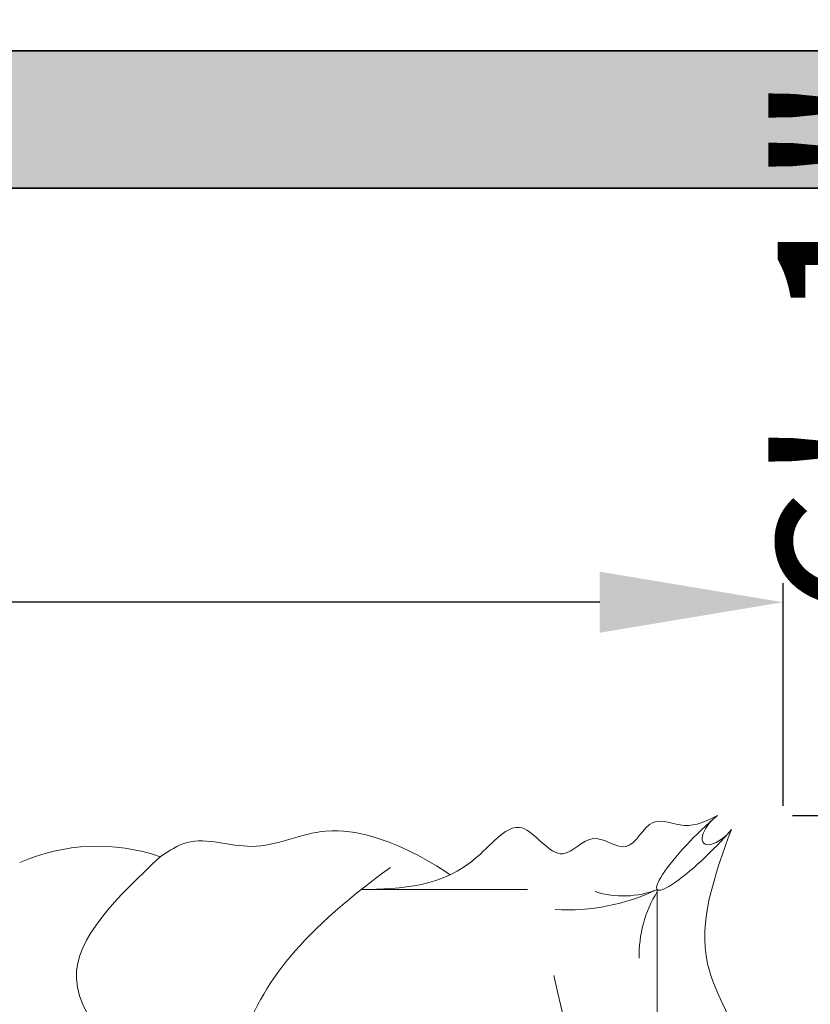
# Model space of a CAD drawing. Units: inches. Extents: x 2083 to 3317, y 1141 to 2115.
# Tile 99 of 256: x 2287 to 2339, y 1958 to 2023. Entities that reach past the tile are written whole.
import ezdxf

# ---------------------------------------------------------------- set-up
doc = ezdxf.new("R2010")
doc.units = ezdxf.units.IN
for name, color, linetype, lineweight in [('A-ANNO-DIMS', 2, 'Continuous', 18), ('A-FURN', 8, 'Continuous', 18), ('A-WALL', 7, 'Continuous', 35), ('www.cadblocksfree.com', 7, 'Continuous', 9)]:
    doc.layers.add(name, color=color, linetype=linetype, lineweight=lineweight)
doc.layers.add('A-WALL-PATT', color=251, linetype='Continuous', lineweight=13, true_color=0x636466)
doc.styles.get("Standard").update_dxf_attribs({"font": 'arial.ttf'})
doc.dimstyles.new('ISO-25', dxfattribs={"dimtxt": 12, "dimasz": 12, "dimexe": 1.25, "dimexo": 0.625, "dimtad": 1, "dimlunit": 3, "dimtxsty": 'Standard', "dimcen": 2.5, "dimadec": 0, "dimazin": 0, "dimtfac": 1, "dimtmove": 0, "dimatfit": 3, "dimfxl": 1, "dimarcsym": 0})

# ---------------------------------------------------------------- blocks, each defined once
blk = doc.blocks.new('bed')
at = {"layer": 'www.cadblocksfree.com', "ltscale": 0.2}
for p, q in [((3426.379, 1399.908), (3426.379, 1410.814)), ((3363.387, 1391.414), (3426.379, 1391.414))]:
    blk.add_line(p, q, dxfattribs=at)
for centre, radius, start, end in [((3416.575, 1428.082), 12.646, 341.02679, 23.77822), ((3438.819, 1397.314), 13.768, 176.75247, 205.37301), ((3432.135, 1393.639), 6.173, 162.64747, 201.1361), ((3422.111, 1384.801), 7.798, 58.00129, 91.65506)]:
    blk.add_arc(centre, radius, start, end, dxfattribs=at)
for centre, major_axis, ratio, start_param, end_param in [((3429.422, 1388.371), (-3.043, 3.043), 0.168252, 4.250342, 8.316029), ((3430.477, 1387.316), (-1.055, 1.055), 0.453532, 4.422107, 8.144264)]:
    blk.add_ellipse(centre, major_axis=major_axis, ratio=ratio, start_param=start_param, end_param=end_param, dxfattribs=at)
for points, knots in [([(3365.512, 1424.213), (3370.519, 1427.004), (3381.149, 1429.825), (3396.214, 1425.866), (3410.541, 1420.654), (3420.273, 1432.695), (3425.882, 1426.771), (3428.534, 1423.97)], [0.099185, 0.099185, 0.099185, 0.099185, 0.523647, 0.927087, 1.289918, 1.564439, 1.810555, 1.810555, 1.810555, 1.810555]), ([(3428.534, 1423.97), (3428.914, 1423.397), (3430.098, 1421.613), (3428.491, 1417.656), (3430.593, 1413.794), (3429.801, 1409.122), (3428.396, 1406.564), (3427.355, 1404.971)], [0, 0, 0, 0, 0.050513, 0.157399, 0.2842023, 0.3628173, 0.5066917, 0.5066917, 0.5066917, 0.5066917]), ([(3362.057, 1409.866), (3363.638, 1413.65), (3372.978, 1421.337), (3389.682, 1406.045), (3402.396, 1419.984), (3416.037, 1420.167), (3423.233, 1415.231), (3427.827, 1408.899)], [0.029901, 0.029901, 0.029901, 0.029901, 0.276967, 0.797115, 1.093669, 1.464666, 1.788489, 1.788489, 1.788489, 1.788489]), ([(3431.237, 1387.473), (3430.882, 1388.172), (3430.205, 1389.505), (3431.478, 1391.985), (3428.294, 1393.194), (3430.501, 1395.689), (3427.558, 1397.866), (3431.841, 1400.386), (3426.535, 1404.33), (3426.443, 1408.152), (3426.379, 1410.814)], [0, 0, 0, 0, 2.267059, 4.324559, 6.685584, 8.878641, 11.121502, 14.300359, 17.755284, 25.682856, 25.682856, 25.682856, 25.682856]), ([(3368.632, 1397.839), (3375.978, 1400.489), (3385.349, 1402.757), (3397.531, 1395.273), (3413.593, 1410.377), (3407.806, 1395.019), (3420.759, 1398.2)], [0.029901, 0.029901, 0.029901, 0.029901, 0.276967, 0.797115, 1.093669, 1.16836, 1.16836, 1.16836, 1.16836]), ([(3430.32, 1386.556), (3427.327, 1387.653), (3422.148, 1389.55), (3414.529, 1384.137), (3405.607, 1387.046), (3396.29, 1386.314), (3386.838, 1381.282), (3377.742, 1390.272), (3370.778, 1384.799), (3364.626, 1383.966), (3363.275, 1388.265), (3360.778, 1387.151), (3359.446, 1386.556)], [0, 0, 0, 0, 8.93042, 15.449194, 25.485629, 34.878505, 43.598887, 54.554403, 64.16647, 67.461673, 70.610457, 74.213583, 74.213583, 74.213583, 74.213583])]:
    blk.add_open_spline(points, degree=3, knots=knots, dxfattribs=at)
blk = doc.blocks.new('*D20')
at = {"layer": 'A-ANNO-DIMS', "color": 0, "lineweight": -2, "transparency": 16777216}
for p, q in [((2244.15, 1971.316), (2244.15, 1985.902)), ((2337.22, 1971.316), (2337.22, 1985.902)), ((2244.15, 1984.652), (2119.159, 1984.652)), ((2325.22, 1984.652), (2256.15, 1984.652))]:
    blk.add_line(p, q, dxfattribs=at)
at = {"layer": 'A-ANNO-DIMS', "color": 0, "transparency": 16777216}
for points in [[(2256.15, 1986.652), (2256.15, 1982.652), (2244.15, 1984.652)], [(2325.22, 1986.652), (2325.22, 1982.652), (2337.22, 1984.652)]]:
    blk.add_solid(points, dxfattribs=at)
at = {"layer": 'Defpoints', "color": 0, "transparency": 16777216}
for p in [(2244.15, 1984.652), (2244.15, 1970.691), (2337.22, 1970.691)]:
    blk.add_point(p, dxfattribs=at)
at = {"layer": 'A-ANNO-DIMS', "color": 0, "transparency": 16777216, "insert": (2175.654, 1991.404), "char_height": 12, "attachment_point": 5}
blk.add_mtext('BED 7\'-9" TYP.', dxfattribs=at)
blk = doc.blocks.new('*D21')
at = {"layer": 'A-ANNO-DIMS', "color": 0, "lineweight": -2, "transparency": 16777216}
for p, q in [((2351.181, 1970.691), (2351.181, 2057.153)), ((2337.845, 1970.691), (2352.431, 1970.691)), ((2351.181, 1909.744), (2351.181, 1958.691)), ((2337.845, 1897.744), (2352.431, 1897.744))]:
    blk.add_line(p, q, dxfattribs=at)
at = {"layer": 'A-ANNO-DIMS', "color": 0, "transparency": 16777216}
for points in [[(2349.181, 1958.691), (2353.181, 1958.691), (2351.181, 1970.691)], [(2349.181, 1909.744), (2353.181, 1909.744), (2351.181, 1897.744)]]:
    blk.add_solid(points, dxfattribs=at)
at = {"layer": 'Defpoints', "color": 0, "transparency": 16777216}
for p in [(2337.22, 1970.691), (2351.181, 1970.691), (2337.22, 1897.744)]:
    blk.add_point(p, dxfattribs=at)
at = {"layer": 'A-ANNO-DIMS', "color": 0, "transparency": 16777216, "insert": (2344.429, 2019.922), "char_height": 12, "attachment_point": 5, "rotation": 90}
blk.add_mtext('6\'-1" TYP.', dxfattribs=at)
blk = doc.blocks.new('*D36')
at = {"layer": 'A-ANNO-DIMS', "color": 0, "lineweight": -2, "transparency": 16777216}
for p, q in [((2235.96, 2012.386), (2235.96, 2074.361)), ((2471.46, 2012.386), (2471.46, 2074.361)), ((2247.96, 2073.111), (2459.46, 2073.111))]:
    blk.add_line(p, q, dxfattribs=at)
at = {"layer": 'A-ANNO-DIMS', "color": 0, "transparency": 16777216}
for points in [[(2247.96, 2075.111), (2247.96, 2071.111), (2235.96, 2073.111)], [(2459.46, 2075.111), (2459.46, 2071.111), (2471.46, 2073.111)]]:
    blk.add_solid(points, dxfattribs=at)
at = {"layer": 'Defpoints', "color": 0, "transparency": 16777216}
for p in [(2471.46, 2073.111), (2235.96, 2011.761), (2471.46, 2011.761)]:
    blk.add_point(p, dxfattribs=at)
at = {"layer": 'A-ANNO-DIMS', "color": 0, "transparency": 16777216, "insert": (2353.71, 2079.941), "char_height": 12, "attachment_point": 5}
blk.add_mtext('19\'-7 1/2"', dxfattribs=at)

msp = doc.modelspace()

# ---------------------------------------------------------------- hatches: boundary and pattern name
at = {"layer": 'A-WALL-PATT'}
h = msp.add_hatch(color=256, dxfattribs=at)
h.dxf.hatch_style = 1
h.paths.add_polyline_path([(3126.96, 2020.761), (2748.96, 2020.761), (2604.96, 2020.761), (2226.96, 2020.761), (2226.96, 1702.761), (2466.96, 1702.761), (2466.96, 1582.761), (2418.96, 1582.761), (2418.96, 1477.761), (2226.96, 1477.761), (2226.96, 1263.261), (2544.96, 1263.261), (2544.96, 1411.761), (2604.96, 1411.761), (2685.96, 1411.761), (2685.96, 1420.761), (2604.96, 1420.761), (2604.96, 1573.761), (2604.96, 1702.761), (2604.96, 2011.761), (2748.96, 2011.761), (2748.96, 1702.761), (2862.96, 1702.761), (2862.96, 1621.761), (2871.96, 1621.761), (2871.96, 1702.761), (2883.96, 1702.761), (2883.96, 1706.939, -0.026459), (2883.96, 1711.761), (2757.96, 1711.761), (2757.96, 1807.761), (2787.96, 1807.761), (2787.96, 1812.261), (2757.96, 1812.261), (2757.96, 2011.761), (2877.96, 2011.761), (2877.96, 1812.261), (2847.96, 1812.261), (2847.96, 1807.761), (2889.836, 1807.761), (2889.836, 1812.261), (2882.46, 1812.261), (2882.46, 2011.761), (3117.96, 2011.761), (3117.96, 1812.261), (2937.836, 1812.261), (2937.836, 1807.761), (2995.71, 1807.761), (2995.71, 1796.118), (3000.21, 1796.118), (3000.21, 1807.761), (3117.96, 1807.761), (3117.96, 1711.761), (3000.21, 1711.761), (3000.21, 1760.118), (2998.573, 1760.118, -0.020711), (2995.71, 1760.118), (2995.71, 1711.761), (2931.96, 1711.761), (2931.96, 1702.761), (3126.96, 1702.761)])
h.paths.add_polyline_path([(2471.46, 2011.761), (2471.46, 1810.011), (2462.717, 1810.011), (2462.717, 1805.511), (2505.96, 1805.511), (2505.96, 1810.011), (2475.96, 1810.011), (2475.96, 2011.761), (2595.96, 2011.761), (2595.96, 1810.011), (2565.96, 1810.011), (2565.96, 1805.511), (2595.96, 1805.511), (2595.96, 1711.761), (2235.96, 1711.761), (2235.96, 1805.511), (2353.71, 1805.511), (2353.71, 1796.054), (2358.21, 1796.054), (2358.21, 1805.511), (2414.717, 1805.511), (2414.717, 1810.011), (2235.96, 1810.011), (2235.96, 2011.761)], flags=16)
h.paths.add_polyline_path([(2270.205, 1994.61), (2270.205, 1970.61), (2246.205, 1970.61), (2246.205, 1994.61)], flags=0)
edge = h.paths.add_edge_path(flags=0)
edge.add_ellipse((2332.027, 1899.798), major_axis=(-3.043, 3.043), ratio=0.168252, start_angle=-161.33217, end_angle=-156.30711, ccw=False)
edge.add_ellipse((2333.082, 1898.744), major_axis=(-1.055, 1.055), ratio=0.453532, start_angle=-123.37102, end_angle=-94.15911)
edge = h.paths.add_edge_path(flags=0)
edge.add_ellipse((2332.027, 1968.876), major_axis=(3.043, 3.043), ratio=0.168252, start_angle=18.66783, end_angle=23.69289)
edge.add_spline(control_points=[(2332.926, 1970.691), (2332.227, 1970.336), (2330.894, 1969.659), (2328.413, 1970.932), (2327.204, 1967.749), (2324.71, 1969.956), (2322.533, 1967.012), (2320.013, 1971.296), (2317.68, 1968.158), (2316.041, 1967.102), (2315.427, 1966.81)], knot_values=[0, 0, 0, 0, 2.267059, 4.324559, 6.685584, 8.878641, 11.121502, 14.300359, 17.755284, 19.732645, 19.732645, 19.732645, 19.732645], degree=3, periodic=0)
edge.add_ellipse((2332.027, 1968.876), major_axis=(3.043, 3.043), ratio=0.168252, start_angle=18.66783, end_angle=23.69289, ccw=False)
edge.add_ellipse((2333.082, 1969.931), major_axis=(1.055, 1.055), ratio=0.453532, start_angle=56.62898, end_angle=85.84089, ccw=False)
edge = h.paths.add_edge_path(flags=0)
edge.add_spline(control_points=[(2296.428, 1967.988), (2293.628, 1965.336), (2287.704, 1959.727), (2299.744, 1949.996), (2294.533, 1935.669), (2290.573, 1920.604), (2293.394, 1909.974), (2296.185, 1904.967)], knot_values=[0.099185, 0.099185, 0.099185, 0.099185, 0.345301, 0.619822, 0.982653, 1.386093, 1.810555, 1.810555, 1.810555, 1.810555], degree=3, periodic=0)
edge.add_spline(control_points=[(2296.185, 1904.967), (2297.384, 1902.619), (2298.001, 1901.949), (2298.553, 1901.468)], knot_values=[0.006246, 0.006246, 0.006246, 0.006246, 0.055476, 0.055476, 0.055476, 0.055476], degree=3, periodic=0)
edge.add_spline(control_points=[(2298.553, 1901.468), (2297.259, 1900.923), (2295.225, 1900.232), (2293.06, 1900.614), (2292.101, 1900.788), (2292.09, 1900.791)], knot_values=[0.312835, 0.312835, 0.312835, 0.312835, 0.40178, 0.474987, 0.475903, 0.475903, 0.475903, 0.475903], degree=3, periodic=0)
edge.add_arc((2292.794, 1904.664), 3.937, 215.4209, 259.69818, ccw=False)
edge.add_spline(control_points=[(2289.585, 1902.382), (2289.477, 1902.535), (2289.368, 1902.688), (2289.261, 1902.841)], knot_values=[0.102872, 0.102872, 0.102872, 0.102872, 0.116896, 0.116896, 0.116896, 0.116896], degree=3, periodic=0)
edge.add_spline(control_points=[(2289.261, 1902.841), (2288.687, 1902.55), (2287.64, 1902.02), (2285.881, 1901.874), (2283.853, 1901.504), (2281.72, 1899.711), (2278.467, 1899.493), (2276.157, 1901.883), (2272.259, 1899.804), (2267.778, 1901.843), (2262.244, 1900.184), (2257.415, 1901.782), (2254.318, 1900.726), (2253.178, 1900.337)], knot_values=[0, 0, 0, 0, 1.907977, 3.477176, 5.261074, 7.972851, 11.680248, 13.717921, 16.939592, 22.789562, 27.502503, 33.595215, 37.145618, 37.145618, 37.145618, 37.145618], degree=3, periodic=0)
edge.add_line((2253.178, 1900.337), (2250.244, 1902.841))
edge.add_line((2250.244, 1902.841), (2250.244, 1965.833))
edge.add_line((2250.244, 1965.833), (2253.178, 1968.337))
edge.add_spline(control_points=[(2253.178, 1968.337), (2254.318, 1967.948), (2257.415, 1966.892), (2262.244, 1968.49), (2267.778, 1966.831), (2271.527, 1968.537), (2273.876, 1967.828), (2274.207, 1967.728)], knot_values=[0, 0, 0, 0, 0.09018, 0.244935, 0.364644, 0.513233, 0.537855, 0.537855, 0.537855, 0.537855], degree=3, periodic=0)
edge.add_arc((2274.353, 1963.793), 3.937, 72.05113, 92.12795, ccw=False)
edge.add_arc((2281.297, 1985.23), 18.596, 252.05113, 288.56572)
edge.add_arc((2292.317, 1956.029), 12.646, 71.02679, 113.77822, ccw=False)
edge = h.paths.add_edge_path(flags=0)
edge.add_spline(control_points=[(2274.899, 1951.856), (2275.066, 1951.617), (2275.233, 1951.377), (2275.398, 1951.136)], knot_values=[1.409916, 1.409916, 1.409916, 1.409916, 1.43159, 1.43159, 1.43159, 1.43159], degree=3, periodic=0)
edge.add_spline(control_points=[(2275.398, 1951.136), (2275.792, 1950.562), (2276.179, 1949.984), (2276.546, 1949.397)], knot_values=[1.358238, 1.358238, 1.358238, 1.358238, 1.409916, 1.409916, 1.409916, 1.409916], degree=3, periodic=0)
edge.add_line((2276.546, 1949.397), (2277.437, 1947.862))
edge.add_spline(control_points=[(2277.437, 1947.862), (2276.304, 1945.673), (2274.64, 1942.427), (2274.632, 1938.094), (2272.799, 1930.852), (2274.356, 1943.897), (2275.948, 1947.923), (2276.546, 1949.397)], knot_values=[0.005632, 0.005632, 0.005632, 0.005632, 0.186014, 0.266002, 0.357087, 0.59639, 0.739732, 0.739732, 0.739732, 0.739732], degree=3, periodic=0)
edge.add_spline(control_points=[(2276.546, 1949.397), (2276.179, 1949.984), (2275.792, 1950.562), (2275.398, 1951.136)], knot_values=[1.358238, 1.358238, 1.358238, 1.358238, 1.409916, 1.409916, 1.409916, 1.409916], degree=3, periodic=0)
edge.add_spline(control_points=[(2275.398, 1951.136), (2274.943, 1950.08), (2274.208, 1948.025), (2273.935, 1944.851), (2272.469, 1937.627), (2273.466, 1945.696), (2274.701, 1951.059), (2274.899, 1951.856)], knot_values=[0.104364, 0.104364, 0.104364, 0.104364, 0.189636, 0.269624, 0.36071, 0.600013, 0.644622, 0.644622, 0.644622, 0.644622], degree=3, periodic=0)
h.paths.add_polyline_path([(2269.168, 1963.128, -0.357527), (2268.171, 1960.976, -0.092561), (2268.171, 1939.436, -0.357527), (2269.168, 1937.285, -0.357527), (2267.016, 1938.282, -0.164785), (2254.686, 1938.282, -0.357527), (2252.534, 1937.285, -0.357527), (2253.531, 1939.436, -0.092561), (2253.531, 1960.976, -0.357527), (2252.534, 1963.128, -0.357527), (2254.686, 1962.131, -0.164785), (2267.016, 1962.131, -0.357527)], flags=0)
h.paths.add_polyline_path([(2248.874, 1967.802), (2248.874, 1957.028), (2249.458, 1957.028), (2249.458, 1911.647), (2248.874, 1911.647), (2248.874, 1900.873), (2246.512, 1900.873, 0.197327), (2244.15, 1902.457), (2244.15, 1966.218, 0.197327), (2246.512, 1967.802)], flags=0)
h.paths.add_polyline_path([(2269.168, 1931.389, -0.357527), (2268.171, 1929.238, -0.092561), (2268.171, 1907.698, -0.357527), (2269.168, 1905.547, -0.357527), (2267.016, 1906.544, -0.164785), (2254.686, 1906.544, -0.357527), (2252.534, 1905.547, -0.357527), (2253.531, 1907.698, -0.092561), (2253.531, 1929.238, -0.357527), (2252.534, 1931.389, -0.357527), (2254.686, 1930.392, -0.164785), (2267.016, 1930.392, -0.357527)], flags=0)
edge = h.paths.add_edge_path(flags=0)
edge.add_spline(control_points=[(2276.197, 1906.724), (2276.168, 1909.029), (2276.114, 1913.372), (2270.598, 1924.925), (2273.905, 1919.013), (2275.922, 1916.262), (2275.475, 1912.402), (2277.258, 1910.381), (2276.696, 1908.225), (2276.646, 1906.813), (2276.618, 1906.008)], knot_values=[0, 0, 0, 0, 8.61026, 16.221274, 18.843057, 23.804898, 27.440828, 29.356102, 31.203478, 33.650687, 33.650687, 33.650687, 33.650687], degree=3, periodic=0)
edge.add_spline(control_points=[(2276.618, 1906.008), (2276.623, 1905.624), (2276.498, 1904.629), (2275.442, 1903.855), (2274.937, 1903.08), (2274.859, 1902.841)], knot_values=[0.156488, 0.156488, 0.156488, 0.156488, 0.184398, 0.231376, 0.250598, 0.250598, 0.250598, 0.250598], degree=3, periodic=0)
edge.add_line((2274.859, 1902.841), (2276.506, 1902.841))
edge.add_spline(control_points=[(2276.506, 1902.841), (2276.788, 1903.085), (2277.665, 1904.125), (2278.25, 1904.341), (2277.654, 1908.527), (2278.156, 1906.228), (2278.1, 1905.286), (2278.847, 1904.069), (2277.857, 1903.415), (2277.874, 1902.991), (2277.904, 1902.841)], knot_values=[0.059574, 0.059574, 0.059574, 0.059574, 0.080753, 0.103741, 0.16972, 0.176036, 0.207137, 0.240474, 0.262341, 0.27366, 0.27366, 0.27366, 0.27366], degree=3, periodic=0)
edge.add_line((2277.904, 1902.841), (2280.03, 1902.841))
edge.add_spline(control_points=[(2280.03, 1902.841), (2279.888, 1903.088), (2279.499, 1903.982), (2280.152, 1905.939), (2278.104, 1909.658), (2279.762, 1907.185), (2280.328, 1904.875), (2280.485, 1903.49), (2281.463, 1903.249), (2281.758, 1902.936), (2281.834, 1902.841)], knot_values=[0.013856, 0.013856, 0.013856, 0.013856, 0.034874, 0.088867, 0.107879, 0.126738, 0.158714, 0.193757, 0.217487, 0.226722, 0.226722, 0.226722, 0.226722], degree=3, periodic=0)
edge.add_spline(control_points=[(2281.834, 1902.841), (2281.788, 1902.827), (2281.647, 1902.783), (2281.396, 1902.859), (2281.088, 1902.985), (2280.721, 1903.061), (2280.333, 1903.026), (2280.125, 1902.899), (2280.03, 1902.841)], knot_values=[0, 0, 0, 0, 0.14413, 0.435517, 0.749276, 1.153046, 1.548371, 1.878348, 1.878348, 1.878348, 1.878348], degree=3, periodic=0)
edge.add_line((2280.03, 1902.841), (2277.904, 1902.841))
edge.add_spline(control_points=[(2277.904, 1902.841), (2277.893, 1902.796), (2277.865, 1902.68), (2277.607, 1902.687), (2277.274, 1902.801), (2276.838, 1902.62), (2276.584, 1902.789), (2276.506, 1902.841)], knot_values=[0, 0, 0, 0, 0.127189, 0.326199, 0.628009, 1.24357, 1.515331, 1.515331, 1.515331, 1.515331], degree=3, periodic=0)
edge.add_line((2276.506, 1902.841), (2274.859, 1902.841))
edge.add_spline(control_points=[(2274.859, 1902.841), (2274.814, 1902.899), (2274.725, 1903.013), (2274.493, 1903.119), (2274.244, 1902.961), (2273.937, 1903.185), (2273.614, 1902.983), (2273.408, 1902.883), (2273.322, 1902.841)], knot_values=[0, 0, 0, 0, 0.21843, 0.436957, 0.687977, 0.990379, 1.398396, 1.69185, 1.69185, 1.69185, 1.69185], degree=3, periodic=0)
edge.add_spline(control_points=[(2273.322, 1902.841), (2273.617, 1903.446), (2274.274, 1904.538), (2276.027, 1904.574), (2276.207, 1906.584), (2276.197, 1906.724)], knot_values=[0.012227, 0.012227, 0.012227, 0.012227, 0.059472, 0.106218, 0.134458, 0.134458, 0.134458, 0.134458], degree=3, periodic=0)
h.paths.add_polyline_path([(2270.776, 1897.79), (2270.776, 1873.79), (2246.776, 1873.79), (2246.776, 1897.79)], flags=0)
h.paths.add_polyline_path([(2353.71, 1760.005), (2353.71, 1760.054), (2358.21, 1760.054, -0.033729)], flags=0)
h.paths.add_polyline_path([(2321.819, 1737.529), (2341.995, 1737.529, -0.414214), (2343.203, 1736.321), (2343.203, 1721.021, -0.414214), (2341.995, 1719.813), (2321.819, 1719.813, -0.414214), (2320.611, 1721.021), (2320.611, 1736.321, -0.414214)], flags=0)
h.paths.add_polyline_path([(2324.235, 1736.321), (2339.579, 1736.321, -0.414214), (2341.995, 1733.905), (2341.995, 1725.45, -0.414214), (2339.579, 1723.034), (2333.681, 1723.034), (2333.845, 1722.045, -0.870646), (2335.425, 1721.826, -0.767327), (2333.923, 1721.423), (2331.291, 1721.423, -0.767327), (2329.788, 1721.826, -0.870646), (2331.368, 1722.045), (2331.533, 1723.034), (2324.235, 1723.034, -0.414214), (2321.819, 1725.45), (2321.819, 1733.905, -0.414214)], flags=0)
h.paths.add_polyline_path([(2570.484, 1928.615), (2589.684, 1928.615), (2590.169, 1928.615), (2590.169, 1904.993), (2570.484, 1904.993)], flags=0)
h.paths.add_polyline_path([(2574.447, 1927.264, -1), (2572.829, 1927.264, -1)], flags=0)
h.paths.add_polyline_path([(2573.09, 1926.941), (2573.925, 1927.776), (2574.148, 1927.553), (2573.313, 1926.718)], flags=0)
h.paths.add_polyline_path([(2578.779, 1919.73, -1), (2571.592, 1919.73, -1)], flags=0)
h.paths.add_polyline_path([(2578.385, 1919.73, -1), (2571.985, 1919.73, -1)], flags=0)
h.paths.add_polyline_path([(2331.596, 1729.476, -1), (2333.618, 1729.476, -1)], flags=0)
h.paths.add_polyline_path([(2578.034, 1927.264, -1), (2576.416, 1927.264, -1)], flags=0)
h.paths.add_polyline_path([(2576.689, 1927.531), (2576.912, 1927.754), (2577.747, 1926.919), (2577.524, 1926.696)], flags=0)
h.paths.add_polyline_path([(2578.139, 1909.86, -1), (2572.232, 1909.86, -1)], flags=0)
h.paths.add_polyline_path([(2577.745, 1909.86, -1), (2572.625, 1909.86, -1)], flags=0)
h.paths.add_polyline_path([(2583.798, 1927.264, -1), (2582.179, 1927.264, -1)], flags=0)
h.paths.add_polyline_path([(2582.719, 1927.754), (2583.554, 1926.919), (2583.331, 1926.696), (2582.496, 1927.531)], flags=0)
h.paths.add_polyline_path([(2582.496, 1927.531), (2582.719, 1927.754), (2583.554, 1926.919), (2583.331, 1926.696)], flags=0)
h.paths.add_polyline_path([(2587.739, 1920.53, -1), (2581.832, 1920.53, -1)], flags=0)
h.paths.add_polyline_path([(2587.345, 1920.53, -1), (2582.225, 1920.53, -1)], flags=0)
h.paths.add_polyline_path([(2587.385, 1927.264, -1), (2585.766, 1927.264, -1)], flags=0)
h.paths.add_polyline_path([(2586.082, 1926.98), (2586.917, 1927.815), (2587.14, 1927.593), (2586.305, 1926.758)], flags=0)
h.paths.add_polyline_path([(2588.379, 1910.66, -1), (2581.192, 1910.66, -1)], flags=0)
h.paths.add_polyline_path([(2587.985, 1910.66, -1), (2581.585, 1910.66, -1)], flags=0)
h.paths.add_polyline_path([(2417.168, 1729.478), (2437.344, 1729.478, -0.414214), (2438.552, 1728.27), (2438.552, 1712.969, -0.414214), (2437.344, 1711.761), (2417.168, 1711.761, -0.414214), (2415.96, 1712.969), (2415.96, 1728.27, -0.414214)], flags=0)
h.paths.add_polyline_path([(2419.584, 1728.27), (2434.928, 1728.27, -0.414214), (2437.344, 1725.854), (2437.344, 1717.398, -0.414214), (2434.928, 1714.983), (2429.029, 1714.983), (2429.194, 1713.994, -0.870646), (2430.774, 1713.775, -0.767327), (2429.271, 1713.372), (2426.64, 1713.372, -0.767327), (2425.137, 1713.775, -0.870646), (2426.717, 1713.994), (2426.882, 1714.983), (2419.584, 1714.983, -0.414214), (2417.168, 1717.398), (2417.168, 1725.854, -0.414214)], flags=0)
h.paths.add_polyline_path([(2419.584, 1728.27), (2434.928, 1728.27, -0.414214), (2437.344, 1725.854), (2437.344, 1717.398, -0.414214), (2434.928, 1714.983), (2429.029, 1714.983), (2428.358, 1719.009), (2427.553, 1719.009), (2426.882, 1714.983), (2419.584, 1714.983, -0.414214), (2417.168, 1717.398), (2417.168, 1725.854, -0.414214)], flags=0)
h.paths.add_polyline_path([(2426.944, 1721.425, -1), (2428.967, 1721.425, -1)], flags=0)
h.paths.add_polyline_path([(2475.96, 1702.761), (2595.96, 1702.761), (2595.96, 1582.761), (2475.96, 1582.761)], flags=16)
h.paths.add_polyline_path([(2427.96, 1573.761), (2595.96, 1573.761), (2595.96, 1468.761), (2595.96, 1420.761), (2384.46, 1420.761), (2384.46, 1468.761), (2427.96, 1468.761)], flags=16)
h.paths.add_polyline_path([(2379.96, 1468.761), (2379.96, 1420.761), (2235.96, 1420.761), (2235.96, 1468.761)], flags=16)
h.paths.add_polyline_path([(2317.816, 1466.696), (2337.992, 1466.696, -0.414214), (2339.2, 1465.488), (2339.2, 1450.187, -0.414214), (2337.992, 1448.979), (2317.816, 1448.979, -0.414214), (2316.608, 1450.187), (2316.608, 1465.488, -0.414214)], flags=0)
h.paths.add_polyline_path([(2320.232, 1465.488), (2335.576, 1465.488, -0.414214), (2337.992, 1463.072), (2337.992, 1454.616, -0.414214), (2335.576, 1452.2), (2329.677, 1452.2), (2329.842, 1451.212, -0.870646), (2331.422, 1450.992, -0.767327), (2329.92, 1450.59), (2327.288, 1450.59, -0.767327), (2325.785, 1450.992, -0.870646), (2327.365, 1451.212), (2327.53, 1452.2), (2320.232, 1452.2, -0.414214), (2317.816, 1454.616), (2317.816, 1463.072, -0.414214)], flags=0)
h.paths.add_polyline_path([(2320.232, 1465.488), (2335.576, 1465.488, -0.414214), (2337.992, 1463.072), (2337.992, 1454.616, -0.414214), (2335.576, 1452.2), (2329.677, 1452.2), (2329.006, 1456.227), (2328.201, 1456.227), (2327.53, 1452.2), (2320.232, 1452.2, -0.414214), (2317.816, 1454.616), (2317.816, 1463.072, -0.414214)], flags=0)
h.paths.add_polyline_path([(2327.593, 1458.643, -1), (2329.615, 1458.643, -1)], flags=0)
h.paths.add_polyline_path([(2244.412, 1433.34), (2241.921, 1433.34, -0.414214), (2240.018, 1435.244), (2240.018, 1440.953, -0.414211), (2241.921, 1442.856), (2244.412, 1442.856, -1.976472)], flags=0)
h.paths.add_polyline_path([(2245.357, 1434.398, -0.414214), (2245.357, 1441.799, -2.144098)], flags=0)
h.paths.add_polyline_path([(2535.96, 1416.261), (2535.96, 1272.261), (2235.96, 1272.261), (2235.96, 1416.261)], flags=16)
h.paths.add_polyline_path([(2260.12, 1384.293), (2260.12, 1362.039), (2237.865, 1362.039), (2237.865, 1384.293)], flags=0)
edge = h.paths.add_edge_path(flags=0)
edge.add_line((2318.252, 1362.093), (2318.146, 1362.001))
edge.add_ellipse((2317.445, 1360.431), major_axis=(2.822, 2.822), ratio=0.168252, start_angle=18.66783, end_angle=20.94813, ccw=False)
edge.add_ellipse((2318.423, 1361.409), major_axis=(0.978, 0.978), ratio=0.453532, start_angle=56.62898, end_angle=70.2262, ccw=False)
edge = h.paths.add_edge_path(flags=0)
edge.add_line((2319.107, 1295.571), (2319.015, 1295.677))
edge.add_ellipse((2317.445, 1296.378), major_axis=(-2.822, 2.822), ratio=0.168252, start_angle=-161.33217, end_angle=-159.05187, ccw=False)
edge.add_ellipse((2318.423, 1295.4), major_axis=(-0.978, 0.978), ratio=0.453532, start_angle=-123.37102, end_angle=-109.7738)
edge = h.paths.add_edge_path(flags=0)
edge.add_spline(control_points=[(2284.21, 1301.17), (2284.581, 1300.445), (2284.891, 1299.892), (2285.16, 1299.461)], knot_values=[0.039066, 0.039066, 0.039066, 0.039066, 0.055476, 0.055476, 0.055476, 0.055476], degree=3, periodic=0)
edge.add_line((2285.16, 1299.461), (2284.21, 1301.17))
edge = h.paths.add_edge_path(flags=0)
edge.add_line((2280.412, 1297.298), (2283.37, 1297.036))
edge.add_line((2283.37, 1297.036), (2286.406, 1297.926))
edge.add_spline(control_points=[(2286.406, 1297.926), (2285.305, 1297.463), (2284.345, 1297.129), (2283.37, 1297.036)], knot_values=[0.394369, 0.394369, 0.394369, 0.394369, 0.475903, 0.475903, 0.475903, 0.475903], degree=3, periodic=0)
edge.add_spline(control_points=[(2283.37, 1297.036), (2283.281, 1297.028), (2282.316, 1296.957), (2281.313, 1297.134), (2280.423, 1297.296), (2280.412, 1297.298)], knot_values=[0.312835, 0.312835, 0.312835, 0.312835, 0.320246, 0.393453, 0.394369, 0.394369, 0.394369, 0.394369], degree=3, periodic=0)
edge = h.paths.add_edge_path(flags=0)
edge.add_line((2284.436, 1359.607), (2280.446, 1355.328))
edge.add_line((2280.446, 1355.328), (2279.58, 1351.018))
edge.add_line((2279.58, 1351.018), (2282.413, 1346.58))
edge.add_spline(control_points=[(2282.413, 1346.58), (2283.153, 1345.589), (2284.253, 1344.029), (2284.801, 1342.387), (2284.935, 1341.806)], knot_values=[1.240098, 1.240098, 1.240098, 1.240098, 1.332892, 1.382712, 1.382712, 1.382712, 1.382712], degree=3, periodic=0)
edge.add_spline(control_points=[(2284.935, 1341.806), (2285.319, 1340.141), (2285.233, 1338.409), (2284.91, 1336.654)], knot_values=[1.097484, 1.097484, 1.097484, 1.097484, 1.240098, 1.240098, 1.240098, 1.240098], degree=3, periodic=0)
edge.add_spline(control_points=[(2284.91, 1336.654), (2284.587, 1334.899), (2284.027, 1333.12), (2283.463, 1331.361)], knot_values=[0.95487, 0.95487, 0.95487, 0.95487, 1.097484, 1.097484, 1.097484, 1.097484], degree=3, periodic=0)
edge.add_line((2283.463, 1331.361), (2281.89, 1326.153))
edge.add_line((2281.89, 1326.153), (2280.756, 1321.056))
edge.add_line((2280.756, 1321.056), (2280.299, 1316.002))
edge.add_line((2280.299, 1316.002), (2280.716, 1310.95))
edge.add_line((2280.716, 1310.95), (2282.028, 1305.972))
edge.add_line((2282.028, 1305.972), (2284.21, 1301.17))
edge.add_spline(control_points=[(2284.21, 1301.17), (2283.341, 1302.73), (2282.612, 1304.336), (2282.028, 1305.972)], knot_values=[0.099185, 0.099185, 0.099185, 0.099185, 0.241799, 0.241799, 0.241799, 0.241799], degree=3, periodic=0)
edge.add_spline(control_points=[(2282.028, 1305.972), (2281.444, 1307.608), (2281.005, 1309.273), (2280.716, 1310.95)], knot_values=[0.241799, 0.241799, 0.241799, 0.241799, 0.384413, 0.384413, 0.384413, 0.384413], degree=3, periodic=0)
edge.add_spline(control_points=[(2280.716, 1310.95), (2280.433, 1312.588), (2280.289, 1314.277), (2280.299, 1315.962), (2280.299, 1316.002)], knot_values=[0.384413, 0.384413, 0.384413, 0.384413, 0.523647, 0.527028, 0.527028, 0.527028, 0.527028], degree=3, periodic=0)
edge.add_spline(control_points=[(2280.299, 1316.002), (2280.312, 1317.687), (2280.478, 1319.368), (2280.756, 1321.056)], knot_values=[0.527028, 0.527028, 0.527028, 0.527028, 0.669642, 0.669642, 0.669642, 0.669642], degree=3, periodic=0)
edge.add_spline(control_points=[(2280.756, 1321.056), (2281.035, 1322.744), (2281.426, 1324.44), (2281.89, 1326.153)], knot_values=[0.669642, 0.669642, 0.669642, 0.669642, 0.812256, 0.812256, 0.812256, 0.812256], degree=3, periodic=0)
edge.add_spline(control_points=[(2281.89, 1326.153), (2282.264, 1327.533), (2282.788, 1329.262), (2283.353, 1331.018), (2283.463, 1331.361)], knot_values=[0.812256, 0.812256, 0.812256, 0.812256, 0.927087, 0.95487, 0.95487, 0.95487, 0.95487], degree=3, periodic=0)
edge.add_line((2283.463, 1331.361), (2284.91, 1336.654))
edge.add_line((2284.91, 1336.654), (2284.935, 1341.806))
edge.add_line((2284.935, 1341.806), (2282.413, 1346.58))
edge.add_spline(control_points=[(2282.413, 1346.58), (2281.275, 1348.104), (2280.078, 1349.57), (2279.58, 1351.018)], knot_values=[1.382712, 1.382712, 1.382712, 1.382712, 1.525326, 1.525326, 1.525326, 1.525326], degree=3, periodic=0)
edge.add_spline(control_points=[(2279.58, 1351.018), (2279.443, 1351.415), (2279.136, 1352.857), (2279.735, 1354.29), (2280.446, 1355.328)], knot_values=[1.525326, 1.525326, 1.525326, 1.525326, 1.564439, 1.667941, 1.667941, 1.667941, 1.667941], degree=3, periodic=0)
edge.add_spline(control_points=[(2280.446, 1355.328), (2281.426, 1356.758), (2282.931, 1358.183), (2284.436, 1359.607)], knot_values=[1.667941, 1.667941, 1.667941, 1.667941, 1.810555, 1.810555, 1.810555, 1.810555], degree=3, periodic=0)
edge.add_arc((2280.623, 1348.518), 11.726, 71.02679, 113.77822)
edge.add_arc((2270.405, 1375.595), 17.244, 252.05113, 288.56572, ccw=False)
edge.add_arc((2263.966, 1355.718), 3.651, 72.05113, 92.12795)
edge.add_arc((2263.966, 1355.718), 3.651, 92.12795, 177.98513)
edge.add_spline(control_points=[(2260.318, 1355.846), (2260.26, 1354.221), (2260.551, 1350.187), (2262.999, 1346.766), (2264.473, 1344.649)], knot_values=[1.43159, 1.43159, 1.43159, 1.43159, 1.564144, 1.770695, 1.770695, 1.770695, 1.770695], degree=3, periodic=0)
edge.add_line((2264.473, 1344.649), (2264.936, 1343.983))
edge.add_spline(control_points=[(2263.801, 1340.248), (2263.843, 1340.514), (2264.067, 1341.756), (2264.513, 1343.002), (2264.935, 1343.981)], knot_values=[0.53657, 0.53657, 0.53657, 0.53657, 0.559349, 0.644622, 0.644622, 0.644622, 0.644622], degree=3, periodic=0)
edge.add_spline(control_points=[(2264.935, 1343.981), (2265.118, 1343.715), (2265.299, 1343.448), (2265.477, 1343.179)], knot_values=[1.384077, 1.384077, 1.384077, 1.384077, 1.409916, 1.409916, 1.409916, 1.409916], degree=3, periodic=0)
edge.add_spline(control_points=[(2265.477, 1343.179), (2265.655, 1342.911), (2265.829, 1342.641), (2265.999, 1342.369)], knot_values=[1.358238, 1.358238, 1.358238, 1.358238, 1.384077, 1.384077, 1.384077, 1.384077], degree=3, periodic=0)
edge.add_line((2265.999, 1342.369), (2266.826, 1340.946))
edge.add_spline(control_points=[(2266.826, 1340.946), (2268.894, 1337.09), (2271.398, 1325.843), (2270.516, 1310.569), (2275.919, 1301.861), (2277.79, 1299.199)], knot_values=[0.116896, 0.116896, 0.116896, 0.116896, 0.472987, 1.050969, 1.313793, 1.313793, 1.313793, 1.313793], degree=3, periodic=0)
edge.add_spline(control_points=[(2277.79, 1299.199), (2277.839, 1299.128), (2277.889, 1299.057), (2277.94, 1298.987)], knot_values=[0.109884, 0.109884, 0.109884, 0.109884, 0.116896, 0.116896, 0.116896, 0.116896], degree=3, periodic=0)
edge.add_line((2277.94, 1298.987), (2277.789, 1299.199))
edge.add_spline(control_points=[(2277.789, 1299.199), (2277.257, 1298.929), (2276.286, 1298.438), (2275.039, 1298.334), (2274.383, 1298.239), (2274.215, 1298.209)], knot_values=[33.12187, 33.12187, 33.12187, 33.12187, 35.029056, 36.598255, 37.144827, 37.144827, 37.144827, 37.144827], degree=3, periodic=0)
edge.add_line((2274.215, 1298.209), (2273.073, 1297.893))
edge.add_spline(control_points=[(2273.073, 1297.893), (2272.323, 1297.58), (2271.039, 1296.511), (2269.248, 1296.226), (2268.423, 1296.375)], knot_values=[26.532584, 26.532584, 26.532584, 26.532584, 29.198919, 31.839101, 31.839101, 31.839101, 31.839101], degree=3, periodic=0)
edge.add_line((2268.423, 1296.375), (2263.879, 1297.458))
edge.add_spline(control_points=[(2263.879, 1297.458), (2263.556, 1297.359), (2261.86, 1296.839), (2260.239, 1297.282), (2258.933, 1297.516)], knot_values=[15.919551, 15.919551, 15.919551, 15.919551, 16.939592, 21.226067, 21.226067, 21.226067, 21.226067], degree=3, periodic=0)
edge.add_line((2258.933, 1297.516), (2254.055, 1297.329))
edge.add_spline(control_points=[(2254.055, 1297.329), (2253.756, 1297.296), (2252.114, 1297.165), (2250.462, 1297.544), (2249.13, 1297.668)], knot_values=[5.306517, 5.306517, 5.306517, 5.306517, 6.276435, 10.613034, 10.613034, 10.613034, 10.613034], degree=3, periodic=0)
edge.add_line((2249.13, 1297.668), (2244.332, 1296.878))
edge.add_line((2244.332, 1296.878), (2241.611, 1299.199))
edge.add_line((2241.611, 1299.199), (2241.611, 1357.609))
edge.add_line((2241.611, 1357.609), (2244.332, 1359.931))
edge.add_line((2244.332, 1359.931), (2252.729, 1359.543))
edge.add_spline(control_points=[(2252.729, 1359.543), (2252.871, 1359.546), (2253.306, 1359.548), (2253.74, 1359.514), (2254.032, 1359.482)], knot_values=[0.233291, 0.233291, 0.233291, 0.233291, 0.244935, 0.268927, 0.268927, 0.268927, 0.268927], degree=3, periodic=0)
edge.add_line((2254.032, 1359.482), (2259.587, 1359.416))
edge.add_spline(control_points=[(2259.587, 1359.416), (2260.677, 1359.629), (2262.073, 1359.897), (2263.524, 1359.459), (2263.83, 1359.366)], knot_values=[0.422516, 0.422516, 0.422516, 0.422516, 0.513233, 0.537855, 0.537855, 0.537855, 0.537855], degree=3, periodic=0)
edge.add_arc((2263.966, 1355.718), 3.651, 72.05113, 92.12795, ccw=False)
edge.add_arc((2270.405, 1375.595), 17.244, 252.05113, 288.56572)
edge.add_arc((2280.623, 1348.518), 11.726, 71.02679, 113.77822, ccw=False)
h.paths.add_polyline_path([(2240.341, 1359.435), (2240.341, 1349.444), (2240.882, 1349.444), (2240.882, 1307.365), (2240.341, 1307.365), (2240.341, 1297.374), (2238.15, 1297.374, 0.197327), (2235.96, 1298.843), (2235.96, 1357.966, 0.197327), (2238.15, 1359.435)], flags=0)
h.paths.add_polyline_path([(2259.158, 1355.101, -0.357527), (2258.233, 1353.106, -0.092561), (2258.233, 1333.133, -0.357527), (2259.158, 1331.138, -0.357527), (2257.163, 1332.062, -0.164785), (2245.729, 1332.062, -0.357527), (2243.735, 1331.138, -0.357527), (2244.659, 1333.133, -0.092561), (2244.659, 1353.106, -0.357527), (2243.735, 1355.101, -0.357527), (2245.729, 1354.176, -0.164785), (2257.163, 1354.176, -0.357527)], flags=0)
edge = h.paths.add_edge_path(flags=0)
edge.add_line((2265.999, 1342.369), (2266.826, 1340.946))
edge.add_line((2266.826, 1340.946), (2265.308, 1337.814))
edge.add_line((2265.308, 1337.814), (2264.358, 1334.653))
edge.add_line((2264.358, 1334.653), (2264.262, 1333.8))
edge.add_spline(control_points=[(2264.262, 1333.8), (2264.208, 1333.187), (2264.162, 1332.366), (2264.007, 1331.414), (2263.969, 1331.202)], knot_values=[0.464444, 0.464444, 0.464444, 0.464444, 0.516691, 0.531608, 0.531608, 0.531608, 0.531608], degree=3, periodic=0)
edge.add_spline(control_points=[(2263.969, 1331.202), (2263.775, 1330.119), (2263.424, 1328.791), (2263.257, 1328.531), (2263.234, 1328.515)], knot_values=[0.372682, 0.372682, 0.372682, 0.372682, 0.44885, 0.464444, 0.464444, 0.464444, 0.464444], degree=3, periodic=0)
edge.add_spline(control_points=[(2263.234, 1328.515), (2263.096, 1328.42), (2263.131, 1329.301), (2263.275, 1330.616)], knot_values=[0.280919, 0.280919, 0.280919, 0.280919, 0.372682, 0.372682, 0.372682, 0.372682], degree=3, periodic=0)
edge.add_spline(control_points=[(2263.275, 1330.616), (2263.419, 1331.93), (2263.672, 1333.677), (2263.97, 1335.315)], knot_values=[0.189157, 0.189157, 0.189157, 0.189157, 0.280919, 0.280919, 0.280919, 0.280919], degree=3, periodic=0)
edge.add_spline(control_points=[(2263.97, 1335.315), (2264.1, 1336.032), (2264.419, 1337.622), (2264.755, 1338.864), (2264.947, 1339.491)], knot_values=[0.097394, 0.097394, 0.097394, 0.097394, 0.137578, 0.189157, 0.189157, 0.189157, 0.189157], degree=3, periodic=0)
edge.add_spline(control_points=[(2264.947, 1339.491), (2265.29, 1340.606), (2265.644, 1341.494), (2265.999, 1342.369)], knot_values=[0.005632, 0.005632, 0.005632, 0.005632, 0.097394, 0.097394, 0.097394, 0.097394], degree=3, periodic=0)
h.paths.add_polyline_path([(2259.158, 1325.671, -0.357527), (2258.233, 1323.676, -0.092561), (2258.233, 1303.703, -0.357527), (2259.158, 1301.708, -0.357527), (2257.163, 1302.633, -0.164785), (2245.729, 1302.633, -0.357527), (2243.735, 1301.708, -0.357527), (2244.659, 1303.703, -0.092561), (2244.659, 1323.676, -0.357527), (2243.735, 1325.671, -0.357527), (2245.729, 1324.747, -0.164785), (2257.163, 1324.747, -0.357527)], flags=0)
edge = h.paths.add_edge_path(flags=0)
edge.add_spline(control_points=[(2261.709, 1317.311), (2261.679, 1317.418), (2261.762, 1317.389), (2262.491, 1316.09), (2262.962, 1315.301)], knot_values=[14.955861, 14.955861, 14.955861, 14.955861, 16.221274, 18.694826, 18.694826, 18.694826, 18.694826], degree=3, periodic=0)
edge.add_spline(control_points=[(2262.962, 1315.301), (2262.99, 1315.254), (2263.702, 1314.067), (2264.349, 1313.127), (2264.73, 1312.164)], knot_values=[18.694826, 18.694826, 18.694826, 18.694826, 18.843057, 22.433791, 22.433791, 22.433791, 22.433791], degree=3, periodic=0)
edge.add_spline(control_points=[(2264.73, 1312.164), (2264.876, 1311.796), (2265.177, 1310.77), (2265.143, 1309.559), (2265.248, 1308.824)], knot_values=[22.433791, 22.433791, 22.433791, 22.433791, 23.804898, 26.172756, 26.172756, 26.172756, 26.172756], degree=3, periodic=0)
edge.add_line((2265.248, 1308.824), (2265.851, 1307.172))
edge.add_spline(control_points=[(2265.851, 1307.172), (2266.065, 1306.822), (2266.384, 1306.332), (2266.424, 1305.781), (2266.42, 1305.611)], knot_values=[28.062562, 28.062562, 28.062562, 28.062562, 29.356102, 29.911721, 29.911721, 29.911721, 29.911721], degree=3, periodic=0)
edge.add_spline(control_points=[(2266.42, 1305.611), (2266.416, 1305.433), (2266.394, 1305.25), (2266.365, 1305.066)], knot_values=[29.911721, 29.911721, 29.911721, 29.911721, 30.497837, 30.497837, 30.497837, 30.497837], degree=3, periodic=0)
edge.add_line((2266.365, 1305.066), (2266.066, 1302.136))
edge.add_spline(control_points=[(2266.066, 1302.136), (2266.071, 1301.78), (2265.998, 1301.2), (2265.663, 1300.759), (2265.509, 1300.586)], knot_values=[0.156488, 0.156488, 0.156488, 0.156488, 0.184398, 0.203543, 0.203543, 0.203543, 0.203543], degree=3, periodic=0)
edge.add_line((2265.509, 1300.586), (2264.435, 1299.199))
edge.add_line((2264.435, 1299.199), (2265.962, 1299.199))
edge.add_line((2265.962, 1299.199), (2267.336, 1301.175))
edge.add_line((2267.336, 1301.175), (2267.312, 1301.986))
edge.add_spline(control_points=[(2267.312, 1301.986), (2267.261, 1302.862), (2267.16, 1303.737), (2267.271, 1303.326)], knot_values=[0.126229, 0.126229, 0.126229, 0.126229, 0.166617, 0.166617, 0.166617, 0.166617], degree=3, periodic=0)
edge.add_spline(control_points=[(2267.271, 1303.326), (2267.28, 1303.294), (2267.31, 1303.175), (2267.373, 1302.884), (2267.406, 1302.683), (2267.418, 1302.601)], knot_values=[0.166617, 0.166617, 0.166617, 0.166617, 0.16972, 0.176036, 0.180765, 0.180765, 0.180765, 0.180765], degree=3, periodic=0)
edge.add_spline(control_points=[(2267.744, 1300.988), (2267.688, 1301.151), (2267.481, 1301.657), (2267.484, 1302.145), (2267.418, 1302.601)], knot_values=[0.180765, 0.180765, 0.180765, 0.180765, 0.193767, 0.220139, 0.220139, 0.220139, 0.220139], degree=3, periodic=0)
edge.add_line((2267.418, 1302.601), (2267.744, 1300.988))
edge.add_spline(control_points=[(2267.744, 1300.988), (2267.832, 1300.732), (2267.932, 1300.31), (2267.555, 1299.975), (2267.429, 1299.829)], knot_values=[0.220139, 0.220139, 0.220139, 0.220139, 0.240474, 0.25489, 0.25489, 0.25489, 0.25489], degree=3, periodic=0)
edge.add_line((2267.429, 1299.829), (2267.258, 1299.199))
edge.add_line((2267.258, 1299.199), (2269.23, 1299.199))
edge.add_spline(control_points=[(2269.23, 1299.199), (2269.099, 1299.429), (2268.843, 1300.016), (2269.012, 1300.916), (2268.947, 1301.661)], knot_values=[0.013856, 0.013856, 0.013856, 0.013856, 0.034874, 0.067073, 0.067073, 0.067073, 0.067073], degree=3, periodic=0)
edge.add_line((2268.947, 1301.661), (2268.432, 1303.603))
edge.add_spline(control_points=[(2268.432, 1303.603), (2268.176, 1304.192), (2267.596, 1305.251), (2268.041, 1304.623), (2268.251, 1304.282)], knot_values=[0.090155, 0.090155, 0.090155, 0.090155, 0.107879, 0.120289, 0.120289, 0.120289, 0.120289], degree=3, periodic=0)
edge.add_spline(control_points=[(2268.251, 1304.282), (2268.361, 1304.105), (2269.058, 1302.918), (2269.383, 1301.59), (2269.521, 1300.776), (2269.575, 1300.556)], knot_values=[0.120289, 0.120289, 0.120289, 0.120289, 0.126738, 0.158714, 0.173506, 0.173506, 0.173506, 0.173506], degree=3, periodic=0)
edge.add_line((2269.575, 1300.556), (2270.686, 1299.421))
edge.add_spline(control_points=[(2270.686, 1299.421), (2270.767, 1299.357), (2270.838, 1299.281), (2270.903, 1299.199)], knot_values=[0.21816, 0.21816, 0.21816, 0.21816, 0.226722, 0.226722, 0.226722, 0.226722], degree=3, periodic=0)
edge.add_line((2270.937, 1299.193), (2270.903, 1299.199))
edge.add_spline(control_points=[(2270.903, 1299.199), (2270.86, 1299.186), (2270.73, 1299.146), (2270.496, 1299.216), (2270.272, 1299.308), (2270.121, 1299.348), (2270.063, 1299.36)], knot_values=[0.939174, 0.939174, 0.939174, 0.939174, 1.083304, 1.374691, 1.68845, 1.878348, 1.878348, 1.878348, 1.878348], degree=3, periodic=0)
edge.add_line((2270.063, 1299.36), (2269.23, 1299.199))
edge.add_line((2269.23, 1299.199), (2267.258, 1299.199))
edge.add_spline(control_points=[(2267.258, 1299.199), (2267.248, 1299.157), (2267.223, 1299.05), (2266.984, 1299.057), (2266.809, 1299.116), (2266.677, 1299.109), (2266.637, 1299.105)], knot_values=[0.757665, 0.757665, 0.757665, 0.757665, 0.884854, 1.083864, 1.385675, 1.515331, 1.515331, 1.515331, 1.515331], degree=3, periodic=0)
edge.add_spline(control_points=[(2266.637, 1299.105), (2266.485, 1299.089), (2266.236, 1299.017), (2266.035, 1299.151), (2265.962, 1299.199)], knot_values=[0, 0, 0, 0, 0.485905, 0.757665, 0.757665, 0.757665, 0.757665], degree=3, periodic=0)
edge.add_line((2265.962, 1299.199), (2264.435, 1299.199))
edge.add_line((2264.435, 1299.199), (2263.858, 1299.367))
edge.add_spline(control_points=[(2263.858, 1299.367), (2263.819, 1299.371), (2263.78, 1299.386), (2263.74, 1299.402)], knot_values=[0.845925, 0.845925, 0.845925, 0.845925, 0.978627, 0.978627, 0.978627, 0.978627], degree=3, periodic=0)
edge.add_line((2263.722, 1299.396), (2263.01, 1299.199))
edge.add_spline(control_points=[(2263.01, 1299.199), (2263.246, 1299.683), (2263.506, 1300.128), (2263.873, 1300.408)], knot_values=[0.012227, 0.012227, 0.012227, 0.012227, 0.052971, 0.052971, 0.052971, 0.052971], degree=3, periodic=0)
edge.add_spline(control_points=[(2263.873, 1300.408), (2263.932, 1300.453), (2264.084, 1300.553), (2264.255, 1300.624), (2264.36, 1300.665)], knot_values=[0.052971, 0.052971, 0.052971, 0.052971, 0.059472, 0.069086, 0.069086, 0.069086, 0.069086], degree=3, periodic=0)
edge.add_line((2264.36, 1300.665), (2265.142, 1301.078))
edge.add_line((2265.142, 1301.078), (2265.676, 1302.8))
edge.add_line((2265.676, 1302.8), (2265.541, 1305.704))
edge.add_line((2265.541, 1305.704), (2264.803, 1309.328))
edge.add_line((2264.803, 1309.328), (2263.041, 1314.092))
edge.add_spline(control_points=[(2263.041, 1314.092), (2262.384, 1315.671), (2261.796, 1316.998), (2261.709, 1317.311)], knot_values=[11.216896, 11.216896, 11.216896, 11.216896, 14.955861, 14.955861, 14.955861, 14.955861], degree=3, periodic=0)
h.paths.add_polyline_path([(2871.96, 1416.261), (2895.91, 1416.261), (2895.91, 1420.761), (2871.96, 1420.761), (2871.96, 1501.761), (2862.96, 1501.761), (2862.96, 1420.761), (2805.96, 1420.761), (2805.96, 1411.761), (2862.96, 1411.761), (2862.96, 1263.261), (3126.96, 1263.261), (3126.96, 1411.761), (3126.96, 1486.761), (2943.96, 1486.761), (2943.96, 1477.761), (2967.86, 1477.761), (2967.86, 1420.761), (2943.91, 1420.761), (2943.91, 1416.261), (3117.96, 1416.261), (3117.96, 1420.761), (2972.36, 1420.761), (2972.36, 1477.761), (3117.96, 1477.761), (3117.96, 1420.761), (3117.96, 1272.261), (2871.96, 1272.261)], flags=0)
h.paths.add_polyline_path([(2457.126, 1485.943), (2527.603, 1485.943), (2527.603, 1537.636), (2457.126, 1537.636)], flags=8)
h.paths.add_polyline_path([(2481.005, 1609.982), (2590.766, 1609.982), (2590.766, 1682.003), (2481.005, 1682.003)], flags=8)
h.paths.add_polyline_path([(2483.085, 1729.127), (2553.562, 1729.127), (2553.562, 1780.82), (2483.085, 1780.82)], flags=8)

# ---------------------------------------------------------------- linework, layer by layer
at = {"layer": 'A-WALL'}
for p, q in [((2226.96, 2020.761), (2604.96, 2020.761)), ((2235.96, 2011.761), (2471.46, 2011.761))]:
    msp.add_line(p, q, dxfattribs=at)

# ---------------------------------------------------------------- block references
at = {"layer": 'A-FURN', "rotation": 90}
msp.add_blockref('bed', (3720.398, -1460.546), dxfattribs=at)

# ---------------------------------------------------------------- dimensions: what is measured, and where the dimension line sits
at = {"layer": 'A-ANNO-DIMS'}
dim = msp.add_linear_dim(base=(2471.46, 2073.111), p1=(2235.96, 2011.761), p2=(2471.46, 2011.761), dimstyle='ISO-25', override={"dimdec": 1, "dimlfac": 1, "dimrnd": 0, "dimzin": 1, "dimdsep": 46, "dimlunit": 4, "dimfrac": 2}, dxfattribs=at)
dim.commit()
dim.dimension.update_dxf_attribs({"geometry": '*D36', "text_midpoint": (2353.71, 2079.941)})
for base, p1, p2, angle, text, picture, middle in [((2351.181, 1970.691), (2337.22, 1897.744), (2337.22, 1970.691), 90, '<> TYP.', '*D21', (2344.429, 2019.922)), ((2244.15, 1984.652), (2337.22, 1970.691), (2244.15, 1970.691), 180, 'BED <> TYP.', '*D20', (2175.654, 1991.404))]:
    dim = msp.add_linear_dim(base=base, p1=p1, p2=p2, angle=angle, text=text, dimstyle='ISO-25', override={"dimdec": 1, "dimlfac": 1, "dimrnd": 0, "dimzin": 1, "dimdsep": 46, "dimlunit": 4, "dimfrac": 2}, dxfattribs=at)
    dim.commit()
    dim.dimension.update_dxf_attribs({"geometry": picture, "text_midpoint": middle})

doc.saveas('drawing.dxf')
